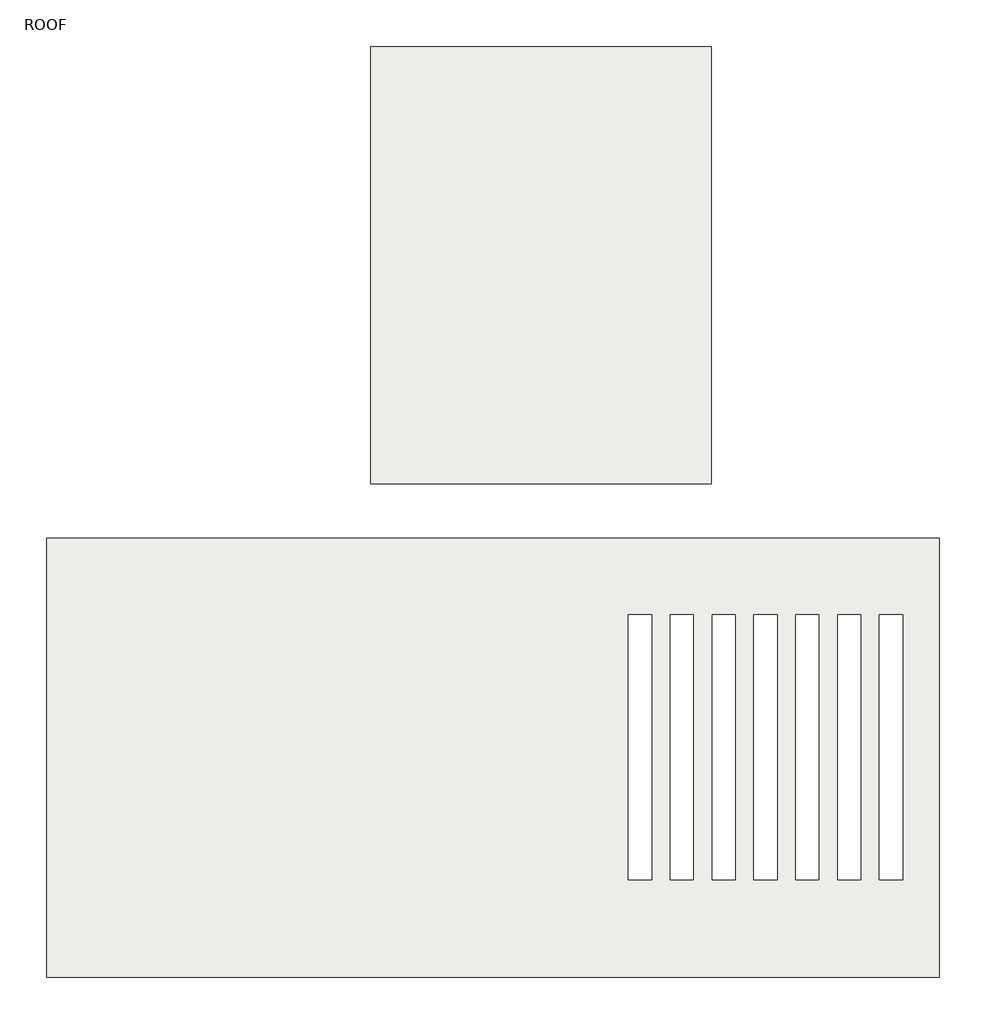
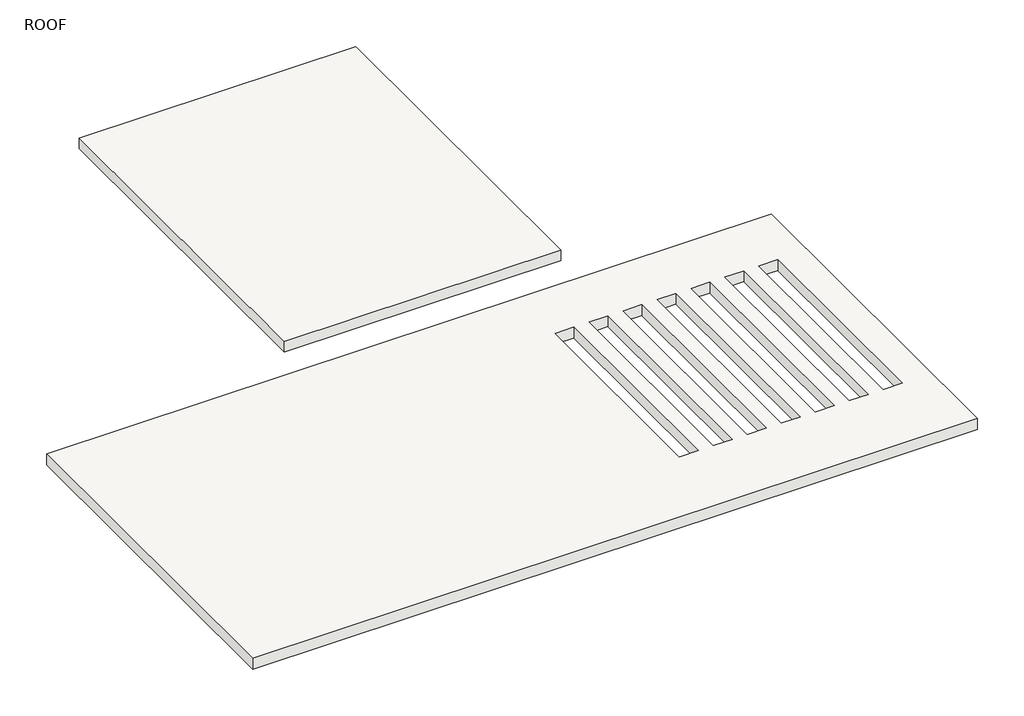
# One storey: 2 slabs.
"""IFC4 building model written with IfcOpenShell, lengths in millimetres."""

from ifc_helpers import new_model, si_unit, frame, origin, place, context, project, spatial, polyline, outline, extrude, element, save

model = new_model("IFC4")

# Units and contexts
model_context = context("Model", 3, world=origin())
ifc_project = project(units=[si_unit("LENGTHUNIT", "METRE", prefix="MILLI")], contexts=[model_context])

# Site, building, storey
site = spatial("IfcSite", under=ifc_project)
building = spatial("IfcBuilding", under=site)
storey = spatial("IfcBuildingStorey", under=building, Name="ROOF", Elevation=9601.2)

# Slabs
placement = place(None, origin())
element("IfcSlab", 1, ObjectType="6\"", at=placement, inside=storey, context=model_context, shape_type="SweptSolid", body=[
    extrude(outline(polyline([(827.5584916, 4005.2935985), (827.5584916, -771.4533727), (-2893.5415084, -771.4533727), (-2893.5415084, 4005.2935985), (827.5584916, 4005.2935985)])), frame((0.0, 0.0, 9448.8), z_axis=(0.0, 0.0, 1.0), x_axis=(1.0, 0.0, 0.0)), (0.0, 0.0, 1.0), 152.4),
])
element("IfcSlab", 2, ObjectType="6\"", at=placement, inside=storey, context=model_context, shape_type="SweptSolid", body=[
    extrude(outline(polyline([(-6436.8415084, -6167.4064015), (-6436.8415084, -1366.8064015), (3316.7584916, -1366.8064015), (3316.7584916, -6167.4064015), (-6436.8415084, -6167.4064015)]), holes=[polyline([(175.4825935, -2205.0064015), (-78.5174065, -2205.0064015), (-78.5174065, -5102.2529878), (175.4825935, -5102.2529878), (175.4825935, -2205.0064015)]), polyline([(632.6825935, -2205.0064015), (378.6825935, -2205.0064015), (378.6825935, -5102.2529878), (632.6825935, -5102.2529878), (632.6825935, -2205.0064015)]), polyline([(1089.8825935, -2205.0064015), (835.8825935, -2205.0064015), (835.8825935, -5102.2529878), (1089.8825935, -5102.2529878), (1089.8825935, -2205.0064015)]), polyline([(1547.0825935, -2205.0064015), (1293.0825935, -2205.0064015), (1293.0825935, -5102.2529878), (1547.0825935, -5102.2529878), (1547.0825935, -2205.0064015)]), polyline([(2004.2825935, -2205.0064015), (1750.2825935, -2205.0064015), (1750.2825935, -5102.2529878), (2004.2825935, -5102.2529878), (2004.2825935, -2205.0064015)]), polyline([(2461.4825935, -2205.0064015), (2207.4825935, -2205.0064015), (2207.4825935, -5102.2529878), (2461.4825935, -5102.2529878), (2461.4825935, -2205.0064015)]), polyline([(2918.6825935, -2205.0064015), (2664.6825935, -2205.0064015), (2664.6825935, -5102.2529878), (2918.6825935, -5102.2529878), (2918.6825935, -2205.0064015)])]), frame((0.0, 0.0, 9448.8), z_axis=(0.0, 0.0, 1.0), x_axis=(1.0, 0.0, 0.0)), (0.0, 0.0, 1.0), 152.4),
])

save(model, "model.ifc")

# Revit data of these elements
# Type "6\""
#   Assembly Code = "B1010"
#   Function = 0
#   Layers, outside or top first: 0' - 6" no material (function 1)
# Element 1 (IfcSlab, "6\"")
#   Height Offset From Level = 0' - 0"
#   Phase Created = New Construction
#   Materials on its faces: "wall 2", "Default Floor"
# Element 2 (IfcSlab, "6\"")
#   Height Offset From Level = 0' - 0"
#   Phase Created = New Construction
#   Materials on its faces: "Default Floor", "wall 2"
# Materials
#   "wall 2": class "Generic", colour RGB 66 64 54, transparency 0, Cost = 0
#   "Default Floor": colour RGB 128 128 128, transparency 0, Cost = 0
